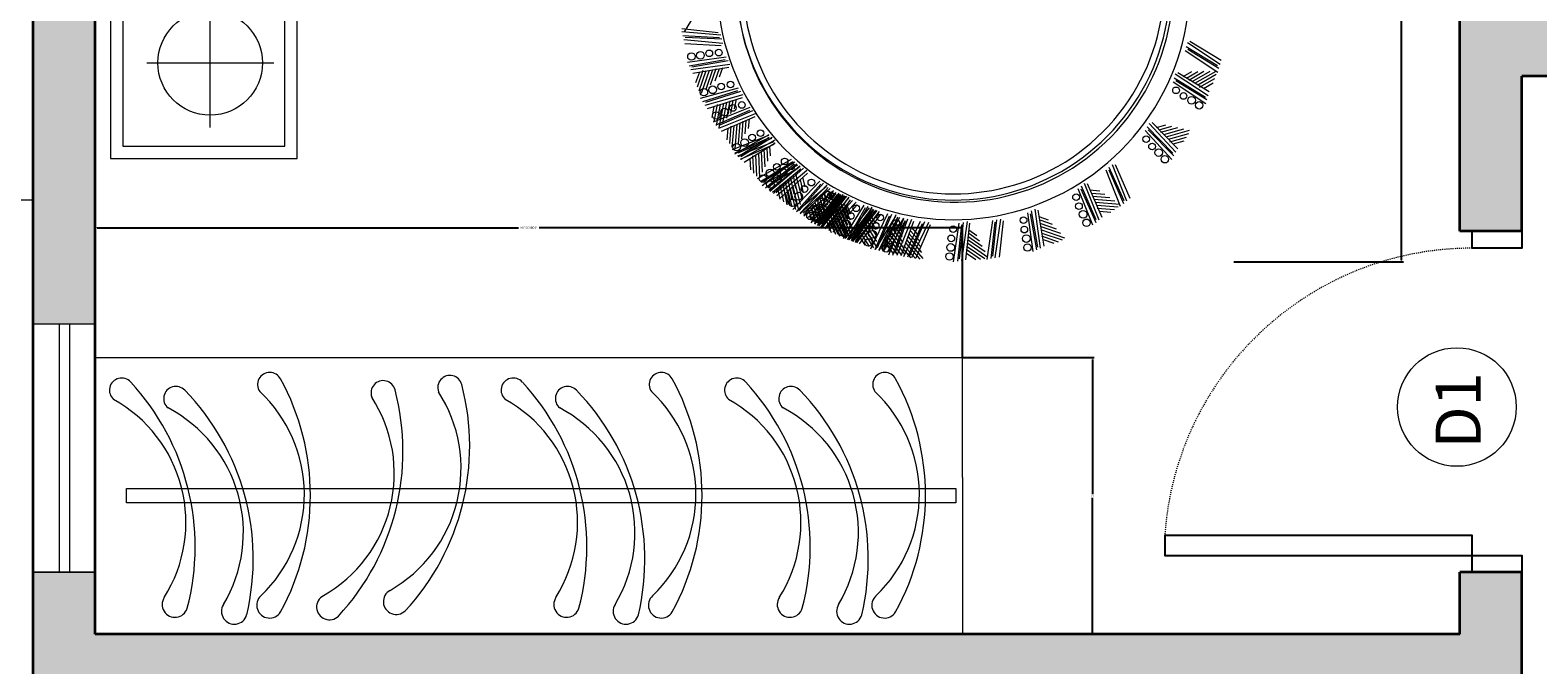
# Model space of a CAD drawing. Units: inches. Extents: x 2701 to 6846, y 811 to 2447.
# Tile 9 of 20: x 2780 to 2926, y 1309 to 1371. Entities that reach past the tile are written whole.
import ezdxf

# ---------------------------------------------------------------- set-up
doc = ezdxf.new("R2010")
doc.units = ezdxf.units.IN
doc.linetypes.add('HIDDEN4', pattern=[0.09375, 0.0625, -0.03125])
for name, color, linetype, lineweight in [('A-ANNO-DIMS', 2, 'Continuous', 18), ('A-ANNO-IDEN', 7, 'Continuous', 13), ('A-DOOR', 4, 'Continuous', 25), ('A-DOOR-SWNG', 4, 'HIDDEN4', 13), ('A-FLOR-PATT', 252, 'Continuous', 13), ('A-FURN', 8, 'Continuous', 13), ('A-GLAZ', 4, 'Continuous', 18), ('A-WALL', 7, 'Continuous', 35)]:
    doc.layers.add(name, color=color, linetype=linetype, lineweight=lineweight)
doc.layers.add('A-WALL-PATT', color=18, linetype='Continuous', lineweight=13, true_color=0x000000)
doc.styles.add('DIM_FONT', font='SIMPLEX.shx', dxfattribs={"width": 0.8})
doc.styles.get("Standard").update_dxf_attribs({"font": 'arial.ttf'})
doc.dimstyles.get("Standard").update_dxf_attribs({"dimtxt": 0.18, "dimasz": 0.18, "dimexe": 0.18, "dimexo": 0.0625, "dimgap": 0.09, "dimtad": 0, "dimtih": 1, "dimtoh": 1, "dimdec": 4, "dimzin": 0, "dimdsep": 46, "dimtxsty": 'Standard', "dimcen": 0.09, "dimadec": 0, "dimazin": 0, "dimtfac": 1, "dimtdec": 4, "dimtofl": 0, "dimtmove": 0, "dimatfit": 3, "dimfxl": 1, "dimtolj": 1, "dimtzin": 0, "dimarcsym": 0})

# ---------------------------------------------------------------- blocks, each defined once
blk = doc.blocks.new('A$C187B6359')
for p, q in [((0.2493, 2.7052), (0.2493, 2.2552)), ((0.6993, 2.7052), (0.2493, 2.7052)), ((0.2793, 2.6752), (0.2793, 2.2852)), ((0.6693, 2.6752), (0.2793, 2.6752)), ((0.4797, 2.6178), (0.4797, 2.3115)), ((0.3236, 2.4648), (0.6327, 2.4648)), ((0.2493, 2.2552), (0.6993, 2.2552)), ((0.2793, 2.2852), (0.6693, 2.2852)), ((0.4729, 1.3107), (0.4877, 1.2238)), ((0.4818, 1.3151), (0.4943, 1.2215)), ((0.5264, 1.3215), (0.5217, 1.2334)), ((0.5361, 1.3238), (0.5277, 1.2297)), ((0.5421, 1.3201), (0.5374, 1.232)), ((0.5458, 1.3261), (0.5411, 1.238)), ((0.5555, 1.3284), (0.5471, 1.2343)), ((0.5629, 1.3285), (0.5533, 1.2408)), ((0.6047, 1.292), (0.5545, 1.3229)), ((0.3781, 1.2719), (0.4034, 1.1809)), ((0.3863, 1.2774), (0.413, 1.1934)), ((0.3946, 1.283), (0.4199, 1.192)), ((0.4617, 1.2625), (0.406, 1.2816)), ((0.4604, 1.2704), (0.4117, 1.2871)), ((0.4614, 1.2774), (0.4216, 1.2911)), ((0.4577, 1.2862), (0.4318, 1.2951)), ((0.455, 1.302), (0.4698, 1.215)), ((0.4639, 1.3064), (0.4764, 1.2128)), ((0.4706, 1.3041), (0.4854, 1.2171)), ((0.3226, 1.2389), (0.3575, 1.1512)), ((0.3819, 1.2281), (0.3242, 1.2393)), ((0.3795, 1.2357), (0.3291, 1.2455)), ((0.3296, 1.2383), (0.3651, 1.1576)), ((0.3302, 1.2453), (0.3657, 1.1646)), ((0.3378, 1.2518), (0.3728, 1.164)), ((0.3796, 1.2429), (0.3383, 1.2509)), ((0.3747, 1.251), (0.3478, 1.2562)), ((0.3698, 1.2663), (0.3965, 1.1822)), ((0.385, 1.2705), (0.4116, 1.1864)), ((0.4631, 1.2546), (0.4159, 1.2708)), ((0.4656, 1.2462), (0.4257, 1.2599)), ((0.4657, 1.2388), (0.4355, 1.2491)), ((0.4677, 1.2306), (0.4454, 1.2383)), ((0.2607, 1.2004), (0.3074, 1.1183)), ((0.2632, 1.1997), (0.2988, 1.1189)), ((0.2708, 1.2061), (0.3058, 1.1184)), ((0.3311, 1.1958), (0.2725, 1.2008)), ((0.3279, 1.2031), (0.2767, 1.2075)), ((0.3272, 1.2103), (0.2853, 1.2138)), ((0.3214, 1.2178), (0.2942, 1.2201)), ((0.315, 1.2325), (0.3505, 1.1518)), ((0.3844, 1.2204), (0.3354, 1.23)), ((0.388, 1.2125), (0.3466, 1.2206)), ((0.3892, 1.2052), (0.3578, 1.2113)), ((0.3923, 1.1974), (0.3691, 1.2019)), ((0.2492, 1.1645), (0.2218, 1.163)), ((0.2407, 1.1781), (0.2871, 1.1031)), ((0.2474, 1.1856), (0.2941, 1.1035)), ((0.248, 1.1868), (0.2836, 1.1061)), ((0.254, 1.193), (0.3004, 1.1179)), ((0.2544, 1.1859), (0.3008, 1.1109)), ((0.2556, 1.1933), (0.2906, 1.1055)), ((0.2626, 1.1927), (0.2982, 1.1119)), ((0.3344, 1.1885), (0.2846, 1.1927)), ((0.3389, 1.181), (0.2968, 1.1846)), ((0.3408, 1.1738), (0.309, 1.1765)), ((0.3447, 1.1664), (0.3212, 1.1684)), ((0.1789, 1.1264), (0.2352, 1.0585)), ((0.1845, 1.1347), (0.2421, 1.0599)), ((0.1874, 1.1311), (0.2341, 1.049)), ((0.194, 1.1385), (0.2404, 1.0634)), ((0.1944, 1.1315), (0.2408, 1.0564)), ((0.2007, 1.1459), (0.2474, 1.0638)), ((0.2618, 1.144), (0.203, 1.1409)), ((0.2576, 1.1509), (0.2063, 1.1481)), ((0.2559, 1.1578), (0.2139, 1.1555)), ((0.266, 1.1372), (0.2162, 1.1345)), ((0.2715, 1.1305), (0.2294, 1.1282)), ((0.1856, 1.0919), (0.1444, 1.0838)), ((0.178, 1.0976), (0.1512, 1.0923)), ((0.1547, 1.0907), (0.2141, 1.0255)), ((0.1599, 1.0992), (0.2209, 1.0271)), ((0.1651, 1.1077), (0.2244, 1.0425)), ((0.1667, 1.1009), (0.2261, 1.0356)), ((0.1678, 1.1099), (0.2241, 1.042)), ((0.1703, 1.1162), (0.2313, 1.0441)), ((0.1733, 1.1182), (0.231, 1.0434)), ((0.1802, 1.1195), (0.2366, 1.0516)), ((0.1807, 1.1237), (0.2271, 1.0486)), ((0.2744, 1.1236), (0.2425, 1.1218)), ((0.2793, 1.1168), (0.2557, 1.1155)), ((0.1817, 1.0611), (0.1245, 1.0471)), ((0.1261, 1.0612), (0.1943, 0.9959)), ((0.1763, 1.067), (0.1264, 1.0548)), ((0.1734, 1.0735), (0.1325, 1.0636)), ((0.1934, 1.0791), (0.1356, 1.0678)), ((0.1882, 1.0852), (0.1378, 1.0754)), ((0.1871, 1.0551), (0.1386, 1.0433)), ((0.1655, 1.0789), (0.1389, 1.0724)), ((0.1985, 1.0729), (0.1495, 1.0633)), ((0.2049, 1.067), (0.1634, 1.0589)), ((0.2087, 1.0605), (0.1774, 1.0544)), ((0.2145, 1.0545), (0.1913, 1.05)), ((0.1337, 1.0191), (0.0941, 1.0049)), ((0.1253, 1.0235), (0.0995, 1.0143)), ((0.1057, 1.0262), (0.1651, 0.9609)), ((0.1109, 1.0347), (0.1719, 0.9626)), ((0.1133, 1.0342), (0.1792, 0.9755)), ((0.1161, 1.0432), (0.1754, 0.9779)), ((0.1176, 1.0432), (0.1858, 0.9779)), ((0.1178, 1.0363), (0.1771, 0.9711)), ((0.1213, 1.0517), (0.1823, 0.9796)), ((0.1218, 1.0522), (0.1877, 0.9935)), ((0.1242, 1.0456), (0.1901, 0.9869)), ((0.1937, 1.0495), (0.1527, 1.0395)), ((0.1979, 1.0433), (0.1668, 1.0357)), ((0.2039, 1.0375), (0.181, 1.0319)), ((0.0799, 0.9828), (0.1458, 0.9242)), ((0.0814, 0.983), (0.1561, 0.9253)), ((0.0835, 0.9891), (0.1533, 0.9352)), ((0.0842, 0.9918), (0.1524, 0.9266)), ((0.0847, 0.9924), (0.1563, 0.941)), ((0.0847, 0.9891), (0.1588, 0.9306)), ((0.0871, 0.9983), (0.1598, 0.938)), ((0.0877, 0.9861), (0.1594, 0.9347)), ((0.1433, 1.0075), (0.0879, 0.9877)), ((0.0879, 1.0018), (0.1627, 0.9441)), ((0.088, 0.9985), (0.1592, 0.9463)), ((0.1373, 1.0129), (0.0889, 0.9955)), ((0.0907, 1.0076), (0.1605, 0.9537)), ((0.091, 0.9921), (0.1622, 0.94)), ((0.0914, 1.0078), (0.1656, 0.9493)), ((0.0935, 1.0012), (0.1634, 0.9473)), ((0.0943, 1.0169), (0.167, 0.9566)), ((0.1493, 1.0022), (0.1023, 0.9854)), ((0.1564, 0.9973), (0.1167, 0.9831)), ((0.1612, 0.9915), (0.1312, 0.9808)), ((0.1678, 0.9864), (0.1456, 0.9784)), ((0.1107, 0.9503), (0.0577, 0.9247)), ((0.1042, 0.9549), (0.0579, 0.9326)), ((0.1136, 0.956), (0.0603, 0.931)), ((0.1071, 0.9608), (0.0606, 0.9389)), ((0.1152, 0.9646), (0.0614, 0.9409)), ((0.1089, 0.9695), (0.0618, 0.9488)), ((0.0999, 0.9607), (0.0621, 0.9424)), ((0.103, 0.9666), (0.0649, 0.9487)), ((0.1049, 0.9754), (0.0664, 0.9585)), ((0.0911, 0.9643), (0.0665, 0.9524)), ((0.0942, 0.9703), (0.0694, 0.9586)), ((0.0962, 0.9793), (0.0711, 0.9683)), ((0.0714, 0.9648), (0.1373, 0.9062)), ((0.1172, 0.9456), (0.0723, 0.9239)), ((0.1201, 0.9513), (0.0749, 0.9301)), ((0.0756, 0.9738), (0.1439, 0.9085)), ((0.1216, 0.9597), (0.0759, 0.9396)), ((0.0781, 0.9736), (0.1498, 0.9222)), ((0.0813, 0.9797), (0.1524, 0.9276)), ((0.0823, 0.9762), (0.1482, 0.9175)), ((0.1277, 0.9471), (0.0895, 0.9292)), ((0.1291, 0.9553), (0.0905, 0.9383)), ((0.1343, 0.9499), (0.105, 0.937)), ((0.1412, 0.9452), (0.1196, 0.9357)), ((0.047, 0.9096), (0.1217, 0.8519)), ((0.0494, 0.9097), (0.1261, 0.8661)), ((0.0495, 0.9161), (0.1236, 0.8576)), ((0.0503, 0.919), (0.122, 0.8676)), ((0.0517, 0.9194), (0.1321, 0.8698)), ((0.0529, 0.9254), (0.124, 0.8733)), ((0.0533, 0.9127), (0.125, 0.8613)), ((0.0535, 0.9284), (0.1283, 0.8707)), ((0.054, 0.9291), (0.1307, 0.8855)), ((0.0559, 0.9191), (0.127, 0.8669)), ((0.0563, 0.9387), (0.1367, 0.8892)), ((0.0563, 0.9348), (0.1304, 0.8763)), ((0.0577, 0.9231), (0.1344, 0.8795)), ((0.1249, 0.9415), (0.0869, 0.9231)), ((0.1302, 0.9362), (0.1015, 0.9224)), ((0.133, 0.9418), (0.1041, 0.9282)), ((0.1373, 0.9318), (0.116, 0.9216)), ((0.1401, 0.9374), (0.1187, 0.9273)), ((0.0314, 0.8727), (0.1166, 0.8319)), ((0.0773, 0.8938), (0.0336, 0.8667)), ((0.0843, 0.8899), (0.0343, 0.8589)), ((0.0725, 0.8991), (0.0368, 0.877)), ((0.0634, 0.9017), (0.0401, 0.8873)), ((0.0437, 0.9002), (0.1154, 0.8488)), ((0.0461, 0.9067), (0.1173, 0.8546)), ((0.0913, 0.8859), (0.0489, 0.8596)), ((0.0993, 0.8826), (0.0635, 0.8604)), ((0.1052, 0.878), (0.0781, 0.8612)), ((0.1127, 0.8744), (0.0927, 0.8619)), ((0.0424, 0.8367), (0.0208, 0.8199)), ((0.0252, 0.8428), (0.1056, 0.7932)), ((0.0275, 0.8525), (0.1042, 0.8089)), ((0.0277, 0.8431), (0.1085, 0.8078)), ((0.0289, 0.8529), (0.1141, 0.8121)), ((0.0298, 0.8621), (0.1102, 0.8126)), ((0.0301, 0.8628), (0.111, 0.8276)), ((0.0312, 0.8465), (0.1079, 0.8029)), ((0.0345, 0.8573), (0.1153, 0.822)), ((0.0151, 0.8), (0.0978, 0.7693)), ((0.0158, 0.8099), (0.1031, 0.774)), ((0.0571, 0.8302), (0.0165, 0.7987)), ((0.0165, 0.8199), (0.0992, 0.7892)), ((0.0171, 0.8298), (0.1045, 0.7938)), ((0.0644, 0.827), (0.0179, 0.7909)), ((0.0517, 0.835), (0.0185, 0.8092)), ((0.0211, 0.8145), (0.1038, 0.7839)), ((0.023, 0.8331), (0.0997, 0.7895)), ((0.0718, 0.8238), (0.0324, 0.7932)), ((0.0801, 0.8214), (0.0468, 0.7955)), ((0.0865, 0.8174), (0.0612, 0.7978)), ((0.0943, 0.8146), (0.0757, 0.8001)), ((0.0452, 0.7888), (0.0064, 0.7551)), ((0.0396, 0.7933), (0.0079, 0.7657)), ((0.0527, 0.7861), (0.0083, 0.7474)), ((0.0094, 0.7641), (0.0902, 0.7289)), ((0.0301, 0.7944), (0.0095, 0.7765)), ((0.0106, 0.774), (0.0958, 0.7332)), ((0.0119, 0.7839), (0.0927, 0.7486)), ((0.0131, 0.7937), (0.0983, 0.7529)), ((0.0162, 0.7783), (0.0971, 0.743)), ((0.0602, 0.7833), (0.0226, 0.7505)), ((0.0687, 0.7813), (0.0369, 0.7536)), ((0.0752, 0.7777), (0.0512, 0.7567)), ((0.0832, 0.7753), (0.0654, 0.7598)), ((0, 0.6734), (0.0935, 0.6598)), ((0.0018, 0.6636), (0.0894, 0.654)), ((0.0075, 0.6596), (0.0952, 0.65)), ((0.0035, 0.6538), (0.097, 0.6402)), ((0.0053, 0.644), (0.093, 0.6344)), ((0.0212, 0.6423), (0.0056, 0.6198)), ((0.0306, 0.6435), (0.0066, 0.609)), ((0.0372, 0.6405), (0.0078, 0.5983)), ((0.0451, 0.6396), (0.0115, 0.5913)), ((0.0531, 0.6388), (0.0246, 0.5978)), ((0.0618, 0.639), (0.0377, 0.6043)), ((0.069, 0.637), (0.0508, 0.6108)), ((0.0774, 0.6367), (0.0639, 0.6173)), ((0.0061, 0.5926), (0.0995, 0.579)), ((0.0078, 0.5828), (0.0955, 0.5732)), ((0.0096, 0.573), (0.1031, 0.5594)), ((0.0113, 0.5632), (0.099, 0.5536)), ((0.0136, 0.5788), (0.1013, 0.5692)), ((0.0247, 0.4821), (0.1183, 0.4946)), ((0.0291, 0.4731), (0.116, 0.4879)), ((0.0334, 0.4642), (0.1271, 0.4767)), ((0.0357, 0.4708), (0.1227, 0.4857)), ((0.0378, 0.4552), (0.1248, 0.47)), ((0.0536, 0.4579), (0.0448, 0.4321)), ((0.0624, 0.4617), (0.0487, 0.4219)), ((0.0694, 0.4606), (0.0528, 0.412)), ((0.0773, 0.462), (0.0582, 0.4063)), ((0.0853, 0.4633), (0.0691, 0.4161)), ((0.0936, 0.4659), (0.0799, 0.426)), ((0.1011, 0.466), (0.0907, 0.4358)), ((0.1092, 0.468), (0.1015, 0.4456)), ((0.0881, 0.3381), (0.1758, 0.373)), ((0.0945, 0.3304), (0.1752, 0.366)), ((0.1015, 0.3299), (0.1822, 0.3654)), ((0.1009, 0.3228), (0.1886, 0.3578)), ((0.1073, 0.3152), (0.188, 0.3508)), ((0.1296, 0.3275), (0.126, 0.2856)), ((0.1367, 0.3282), (0.1323, 0.2769)), ((0.144, 0.3314), (0.139, 0.2727)), ((0.1514, 0.3346), (0.1471, 0.2849)), ((0.1588, 0.3391), (0.1552, 0.2971)), ((0.166, 0.3411), (0.1633, 0.3093)), ((0.1734, 0.345), (0.1714, 0.3214)), ((0.122, 0.3217), (0.1197, 0.2944)), ((0.1337, 0.2711), (0.2215, 0.3061)), ((0.1401, 0.2635), (0.2209, 0.299)), ((0.1466, 0.2559), (0.2343, 0.2908)), ((0.1472, 0.2629), (0.2279, 0.2985)), ((0.153, 0.2483), (0.2337, 0.2838)), ((0.2468, 0.148), (0.3166, 0.2116)), ((0.2555, 0.1431), (0.3185, 0.2048)), ((0.2623, 0.145), (0.3253, 0.2068)), ((0.2642, 0.1382), (0.334, 0.2019)), ((0.2729, 0.1334), (0.3359, 0.1951)), ((0.3243, 0.1845), (0.3307, 0.1618)), ((0.2894, 0.1527), (0.3008, 0.1122)), ((0.2958, 0.1558), (0.3098, 0.1064)), ((0.3015, 0.1614), (0.3176, 0.1048)), ((0.3073, 0.1671), (0.3208, 0.1191)), ((0.3126, 0.1739), (0.3241, 0.1333)), ((0.3187, 0.1783), (0.3274, 0.1475)), ((0.2843, 0.1446), (0.2918, 0.1183)), ((0.3809, 0.0657), (0.4331, 0.1445)), ((0.3906, 0.0631), (0.4366, 0.1384)), ((0.3967, 0.0666), (0.4427, 0.1419)), ((0.4002, 0.0605), (0.4524, 0.1393)), ((0.4098, 0.0579), (0.4559, 0.1332)), ((0.4433, 0.1127), (0.4592, 0.085)), ((0.4472, 0.12), (0.4589, 0.0996)), ((0.4566, 0.0367), (0.5088, 0.1155)), ((0.4662, 0.0341), (0.5123, 0.1094)), ((0.4723, 0.0377), (0.5184, 0.1129)), ((0.4759, 0.0315), (0.528, 0.1103)), ((0.4211, 0.0807), (0.442, 0.0442)), ((0.4265, 0.0853), (0.4522, 0.0407)), ((0.4307, 0.0921), (0.4601, 0.0411)), ((0.4349, 0.099), (0.4598, 0.0557)), ((0.4385, 0.1069), (0.4595, 0.0703)), ((0.4855, 0.029), (0.5315, 0.1042)), ((0.4182, 0.0716), (0.4318, 0.0479))]:
    blk.add_line(p, q)
for centre, radius in [((0.4797, 2.4648), 0.126), ((0.495, 1.3053), 0.00895), ((0.409, 1.2751), 0.00895), ((0.4979, 1.2836), 0.00929), ((0.353, 1.2454), 0.00895), ((0.4149, 1.254), 0.00929), ((0.4227, 1.2335), 0.00801), ((0.5028, 1.2622), 0.00801), ((0.5045, 1.2395), 0.00801), ((0.2766, 1.1962), 0.00895), ((0.3611, 1.2251), 0.00929), ((0.3711, 1.2055), 0.00801), ((0.4275, 1.2112), 0.00801), ((0.2875, 1.1772), 0.00929), ((0.3, 1.1592), 0.00801), ((0.3783, 1.184), 0.00801), ((0.2008, 1.1328), 0.00895), ((0.3101, 1.1388), 0.00801), ((0.1867, 1.1151), 0.00895), ((0.2008, 1.0984), 0.00929), ((0.2142, 1.1155), 0.00929), ((0.2165, 1.083), 0.00801), ((0.2291, 1.0994), 0.00801), ((0.1426, 1.0618), 0.00895), ((0.1584, 1.0467), 0.00929), ((0.2301, 1.0648), 0.00801), ((0.2419, 1.0806), 0.00801), ((0.1078, 1.01), 0.00895), ((0.1107, 1.0186), 0.00895), ((0.1756, 1.033), 0.00801), ((0.1911, 1.0163), 0.00801), ((0.1043, 1.0041), 0.00895), ((0.1216, 0.9908), 0.00929), ((0.1249, 0.9964), 0.00929), ((0.1276, 1.0047), 0.00929), ((0.1401, 0.979), 0.00801), ((0.1434, 0.9844), 0.00801), ((0.1457, 0.9922), 0.00801), ((0.1623, 0.9767), 0.00801), ((0.0722, 0.9428), 0.00895), ((0.1573, 0.964), 0.00801), ((0.1604, 0.9693), 0.00801), ((0.0909, 0.9313), 0.00929), ((0.1106, 0.9215), 0.00801), ((0.1292, 0.9085), 0.00801), ((0.0469, 0.8784), 0.00895), ((0.0666, 0.8689), 0.00929), ((0.0323, 0.8363), 0.00895), ((0.0525, 0.828), 0.00929), ((0.0872, 0.8613), 0.00801), ((0.1071, 0.8503), 0.00801), ((0.0735, 0.8215), 0.00801), ((0.094, 0.8117), 0.00801), ((0.0131, 0.6834), 0.00895), ((0.0347, 0.6803), 0.00929), ((0.0567, 0.6791), 0.00801), ((0.079, 0.6745), 0.00801), ((0.0777, 0.5031), 0.00801), ((0.1003, 0.5048), 0.00801), ((0.0345, 0.4953), 0.00895), ((0.0562, 0.4982), 0.00929), ((0.1147, 0.3614), 0.00929), ((0.1343, 0.3714), 0.00801), ((0.1559, 0.3785), 0.00801), ((0.0944, 0.3533), 0.00895), ((0.2635, 0.1792), 0.00929), ((0.2784, 0.1954), 0.00801), ((0.296, 0.2097), 0.00801), ((0.2474, 0.1644), 0.00895), ((0.4136, 0.1376), 0.00801), ((0.3895, 0.1001), 0.00929), ((0.4, 0.1194), 0.00801), ((0.3775, 0.0818), 0.00895)]:
    blk.add_circle(centre, radius)
for centre, radius, start, end in [((0.6715, 0.6736), 0.5699, 87.1307, 3.1127), ((0.6698, 0.67), 0.5261, 86.7143, 0.065), ((0.6715, 0.6736), 0.5225, 86.8806, 3.3918), ((0.6715, 0.6735), 0.5076, 86.694, 3.4914)]:
    blk.add_arc(centre, radius, start, end)
at = {"style": 'DIM_FONT', "text_generation_flag": 4, "width": 0.8, "flags": 9}
for tag in ['YSIZE', 'XSIZE']:
    blk.add_attdef(tag, (2.1999, 2.7053), '', height=0.0005, rotation=180, dxfattribs=at)
blk = doc.blocks.new('A$C20D7642B')
for p, q in [((0, 1879.7), (0, 0)), ((600, 1879.7), (0, 1879.7)), ((600, 1879.7), (600, 0)), ((285.2, 14), (285.2, 1812.3)), ((285.2, 1812.3), (316, 1812.3)), ((316, 1812.3), (316, 14)), ((340, 0), (0, 0)), ((316, 14), (285.2, 14)), ((340, 0), (600, 0))]:
    blk.add_line(p, q)
for centre, radius, start, end in [((242.6, 1988.3), 305.1, 237.7855, 330.9171), ((529.2, 1822.6), 26.4, 312.0689, 138.8769), ((189.7, 2189.4), 526.2, 255.3064, 312.7492), ((64.5, 1707), 27.8, 56.3378, 252.7376), ((220.7, 1863.8), 305.1, 239.1708, 332.3023), ((511.2, 1705.1), 26.4, 313.4541, 140.2621), ((163, 2063.5), 526.2, 256.6916, 314.1345), ((49.5, 1578.3), 27.8, 57.7231, 254.1228), ((62.8, 1501.9), 27.8, 42.31, 238.7098), ((303.8, 1731.6), 305.1, 223.7577, 316.8893), ((541.6, 1501.4), 26.4, 298.0411, 124.849), ((301.2, 1939.5), 526.2, 241.2786, 298.7214), ((59.1, 1372.1), 27.8, 28.2801, 224.6799), ((348.6, 1536.6), 305.1, 209.7278, 302.8594), ((396.5, 1738.9), 526.2, 227.2487, 284.6915), ((523.6, 1255.6), 26.4, 284.0112, 110.8192), ((70.6, 1227.4), 27.8, 28.2801, 224.6799), ((360, 1391.9), 305.1, 209.7278, 302.8594), ((408, 1594.2), 526.2, 227.2487, 284.6915), ((535, 1110.9), 26.4, 284.0112, 110.8192), ((242.6, 1139.3), 305.1, 237.7855, 330.9171), ((529.2, 973.6), 26.4, 312.0689, 138.8769), ((189.7, 1340.3), 526.2, 255.3064, 312.7492), ((64.5, 857.9), 27.8, 56.3378, 252.7376), ((511.2, 856), 26.4, 313.4541, 140.2621), ((220.7, 1014.8), 305.1, 239.1708, 332.3023), ((163, 1214.5), 526.2, 256.6916, 314.1345), ((49.5, 729.2), 27.8, 57.7231, 254.1228), ((62.8, 652.8), 27.8, 42.31, 238.7098), ((303.8, 882.6), 305.1, 223.7577, 316.8893), ((541.6, 652.4), 26.4, 298.0411, 124.849), ((301.2, 1090.5), 526.2, 241.2786, 298.7214), ((242.6, 655), 305.1, 237.7855, 330.9171), ((529.2, 489.2), 26.4, 312.0689, 138.8769), ((189.7, 856), 526.2, 255.3064, 312.7492), ((64.5, 373.6), 27.8, 56.3378, 252.7376), ((511.2, 371.7), 26.4, 313.4541, 140.2621), ((220.7, 530.5), 305.1, 239.1708, 332.3023), ((163, 730.2), 526.2, 256.6916, 314.1345), ((49.5, 244.9), 27.8, 57.7231, 254.1228), ((62.8, 168.5), 27.8, 42.31, 238.7098), ((303.8, 398.3), 305.1, 223.7577, 316.8893), ((541.6, 168), 26.4, 298.0411, 124.849), ((301.2, 606.1), 526.2, 241.2786, 298.7214)]:
    blk.add_arc(centre, radius, start, end)
blk = doc.blocks.new('DOOR-D1-33IN-PANEL-FRAME')
blk.add_lwpolyline([(0, 33), (0, 31.37), (4.8, 31.37), (4.8, 33), (0, 33)], close=True)
for points in [[(4.32, 33), (0.48, 33)], [(4.8, 0), (4.8, 3.55), (34.54, 3.55), (34.54, 1.63), (0, 1.63), (0, 0)], [(0, 0), (4.8, 0)], [(4.32, 0), (0.48, 0)]]:
    blk.add_lwpolyline(points)
blk = doc.blocks.new('WIN-W2-24IN')
for p, q in [((24, 6), (0, 6)), ((24, 6), (0, 6)), ((0, 0), (0, 6)), ((24, 6), (24, 6)), ((24, 6), (24, 0)), ((24, 3.5), (0, 3.5)), ((24, 2.5), (0, 2.5)), ((24, 0), (0, 0))]:
    blk.add_line(p, q)
blk = doc.blocks.new('*D45')
at = {"layer": 'A-ANNO-DIMS', "color": 0, "lineweight": -2, "transparency": 16777216}
for p, q in [((2785.97, 1338.89), (2785.97, 1351.58)), ((2786.15, 1351.4), (2826.91, 1351.4)), ((2869.67, 1351.4), (2828.91, 1351.4)), ((2869.85, 1338.89), (2869.85, 1351.58))]:
    blk.add_line(p, q, dxfattribs=at)
at = {"layer": 'A-ANNO-DIMS', "color": 0, "transparency": 16777216}
for points in [[(2786.15, 1351.43), (2786.15, 1351.37), (2785.97, 1351.4)], [(2869.67, 1351.43), (2869.67, 1351.37), (2869.85, 1351.4)]]:
    blk.add_solid(points, dxfattribs=at)
at = {"layer": 'Defpoints', "color": 0, "transparency": 16777216}
for p in [(2785.97, 1351.4), (2785.97, 1338.82), (2869.85, 1338.82)]:
    blk.add_point(p, dxfattribs=at)
at = {"layer": 'A-ANNO-DIMS', "color": 0, "transparency": 16777216, "insert": (2827.91, 1351.4), "char_height": 0.18, "attachment_point": 5}
blk.add_mtext('\\A1;WARDROBE 84', dxfattribs=at)
blk = doc.blocks.new('*D46')
at = {"layer": 'A-ANNO-DIMS', "color": 0, "lineweight": -2, "transparency": 16777216}
for p, q in [((2869.91, 1338.82), (2882.61, 1338.82)), ((2882.43, 1338.64), (2882.43, 1325.62)), ((2882.43, 1312.23), (2882.43, 1325.26)), ((2869.91, 1312.05), (2882.61, 1312.05))]:
    blk.add_line(p, q, dxfattribs=at)
at = {"layer": 'A-ANNO-DIMS', "color": 0, "transparency": 16777216}
for points in [[(2882.4, 1338.64), (2882.46, 1338.64), (2882.43, 1338.82)], [(2882.4, 1312.23), (2882.46, 1312.23), (2882.43, 1312.05)]]:
    blk.add_solid(points, dxfattribs=at)
at = {"layer": 'Defpoints', "color": 0, "transparency": 16777216}
for p in [(2869.85, 1338.82), (2882.43, 1338.82), (2869.85, 1312.05)]:
    blk.add_point(p, dxfattribs=at)
at = {"layer": 'A-ANNO-DIMS', "color": 0, "transparency": 16777216, "insert": (2882.43, 1325.44), "char_height": 0.18, "attachment_point": 5}
blk.add_mtext('\\A1;27', dxfattribs=at)
blk = doc.blocks.new('*D50')
at = {"layer": 'A-ANNO-DIMS', "color": 0, "lineweight": -2, "transparency": 16777216}
for p, q in [((2896.11, 1454.53), (2912.52, 1454.53)), ((2912.34, 1454.35), (2912.34, 1401.49)), ((2912.34, 1348.27), (2912.34, 1401.13)), ((2896.11, 1348.09), (2912.52, 1348.09))]:
    blk.add_line(p, q, dxfattribs=at)
at = {"layer": 'A-ANNO-DIMS', "color": 0, "transparency": 16777216}
for points in [[(2912.31, 1454.35), (2912.37, 1454.35), (2912.34, 1454.53)], [(2912.31, 1348.27), (2912.37, 1348.27), (2912.34, 1348.09)]]:
    blk.add_solid(points, dxfattribs=at)
at = {"layer": 'Defpoints', "color": 0, "transparency": 16777216}
for p in [(2896.04, 1454.53), (2912.34, 1454.53), (2896.04, 1348.09)]:
    blk.add_point(p, dxfattribs=at)
at = {"layer": 'A-ANNO-DIMS', "color": 0, "transparency": 16777216, "insert": (2912.34, 1401.31), "char_height": 0.18, "attachment_point": 5}
blk.add_mtext('\\A1;106', dxfattribs=at)

msp = doc.modelspace()

# ---------------------------------------------------------------- hatches: boundary and pattern name
at = {"layer": 'A-FLOR-PATT'}
h = msp.add_hatch(dxfattribs=at)
h.set_pattern_fill('ANGLE', color=256)
h.set_pattern_definition([(0, (0, 0), (0, 6.985), [5.08, -1.905]), (90, (0, 0), (-6.985, 4e-16), [5.08, -1.905])])
h.paths.add_polyline_path([(2841.81, 1296.51, -0.109453), (2842.61, 1300.13, -0.102375), (2844.98, 1303.3, -0.093743), (2848.43, 1305.37, -0.062463), (2851.37, 1306.05), (2785.97, 1306.05), (2785.97, 1258.05), (2827.97, 1258.05), (2827.97, 1256.41), (2829.45, 1256.41, -0.394827), (2854.75, 1283.45), (2856.49, 1283.45), (2856.49, 1256.41), (2857.97, 1256.41), (2857.97, 1258.05), (2863.97, 1258.05), (2863.97, 1306.05), (2853.87, 1306.05, -0.062463), (2856.81, 1305.37, -0.093743), (2860.26, 1303.3, -0.102375), (2862.62, 1300.13, -0.109453), (2863.42, 1296.51, -0.109453), (2862.62, 1292.89, -0.102375), (2860.26, 1289.72, -0.093738), (2856.81, 1287.65, -0.088425), (2852.62, 1286.91, -0.088425), (2848.43, 1287.65, -0.093738), (2844.98, 1289.72, -0.102375), (2842.61, 1292.89, -0.109453)])
h.paths.add_polyline_path([(2805.21, 1273.88, -0.141745), (2808.32, 1271.77, -0.184983), (2809.77, 1267.97, -0.184983), (2808.32, 1264.18, -0.141745), (2805.21, 1262.07, -0.152244), (2799.99, 1261.8, -0.025614), (2799.37, 1261.95), (2794.37, 1263.42), (2794.36, 1263.41, -0.111242), (2793.99, 1261.92, -0.033889), (2793.11, 1260.11, -0.286745), (2792.38, 1259.65), (2787.58, 1259.65, -0.414214), (2787.15, 1260.08), (2787.15, 1267.97), (2787.15, 1275.87, -0.414214), (2787.58, 1276.3), (2792.38, 1276.3, -0.286745), (2793.11, 1275.83, -0.033889), (2793.99, 1274.03, -0.105104), (2794.36, 1272.63), (2794.37, 1272.53), (2799.37, 1274, -0.025614), (2799.99, 1274.15, -0.152244)], flags=16)
h.paths.add_polyline_path([(2804.68, 1272.34, -0.144945), (2807.09, 1270.71, -0.0358), (2807.45, 1270.25, -0.133285), (2807.89, 1268.61), (2807.89, 1267.97), (2807.89, 1267.34, -0.133285), (2807.45, 1265.7, -0.0358), (2807.09, 1265.24, -0.144945), (2804.68, 1263.61, -0.155404), (2800.34, 1263.39, -0.364511), (2796.49, 1267.97, -0.364511), (2800.34, 1272.56, -0.155404)], flags=0)
h.paths.add_polyline_path([(2800.02, 1268.9, 0.169298), (2799.13, 1268.12, 0.076667), (2799.1, 1267.97, 0.076667), (2799.13, 1267.83, 0.169298), (2800.02, 1267.05, 0.305219), (2800.37, 1267.16, 0.169535), (2800.65, 1267.97, 0.169535), (2800.37, 1268.79, 0.305219)], flags=0)
h.paths.add_polyline_path([(2971.97, 1456.05), (2923.97, 1456.05), (2923.97, 1408.05), (2922.33, 1408.05), (2922.33, 1406.57, -0.394827), (2949.37, 1381.27), (2949.37, 1379.53), (2922.33, 1379.53), (2922.33, 1378.05), (2923.97, 1378.05), (2923.97, 1372.05), (2971.97, 1372.05)])
h.paths.add_polyline_path([(2939.82, 1436.53, -0.141745), (2937.71, 1433.42, -0.184983), (2933.91, 1431.97, -0.184983), (2930.12, 1433.42, -0.141745), (2928.01, 1436.53, -0.152244), (2927.74, 1441.75, -0.025614), (2927.89, 1442.37), (2929.36, 1447.38), (2929.35, 1447.38, -0.111242), (2927.86, 1447.75, -0.033889), (2926.05, 1448.63, -0.286745), (2925.59, 1449.37), (2925.59, 1454.16, -0.414214), (2926.02, 1454.59), (2933.91, 1454.59), (2941.81, 1454.59, -0.414207), (2942.24, 1454.16), (2942.24, 1449.37, -0.286745), (2941.78, 1448.63, -0.033889), (2939.97, 1447.75, -0.105104), (2938.57, 1447.38), (2938.47, 1447.38), (2939.94, 1442.37, -0.025614), (2940.09, 1441.75, -0.152244)], flags=16)
h.paths.add_polyline_path([(2938.28, 1437.06, -0.144945), (2936.65, 1434.65, -0.0358), (2936.19, 1434.29, -0.133285), (2934.55, 1433.85), (2933.91, 1433.85), (2933.28, 1433.85, -0.133285), (2931.64, 1434.29, -0.0358), (2931.18, 1434.65, -0.144945), (2929.55, 1437.06, -0.155404), (2929.33, 1441.4, -0.364511), (2933.91, 1445.26, -0.364511), (2938.5, 1441.4, -0.155404)], flags=0)
h.paths.add_polyline_path([(2969.16, 1392.04, -0.093743), (2971.22, 1388.6, -0.088421), (2971.97, 1384.4, -0.088421), (2971.22, 1380.21, -0.093743), (2969.16, 1376.76, -0.102375), (2965.99, 1374.4, -0.109453), (2962.37, 1373.6, -0.109453), (2958.75, 1374.4, -0.102375), (2955.58, 1376.76, -0.093738), (2953.51, 1380.21, -0.088425), (2952.76, 1384.4, -0.088425), (2953.51, 1388.6, -0.093738), (2955.58, 1392.04, -0.102375), (2958.75, 1394.41, -0.109453), (2962.37, 1395.21, -0.109453), (2965.99, 1394.41, -0.102375)], flags=0)
edge = h.paths.add_edge_path(flags=16)
edge.add_arc((2961.07, 1384.86), 10.2, 20.2132, 41.6336, ccw=False)
edge.add_spline(control_points=[(2970.65, 1388.38), (2970.46, 1387.83), (2970, 1386.48), (2971.44, 1384.4), (2969.87, 1382.34), (2970.41, 1381.01), (2970.65, 1380.43)], knot_values=[0, 0, 0, 0, 0.041109, 0.100337, 0.155913, 0.199586, 0.199586, 0.199586, 0.199586], degree=3, periodic=0)
edge.add_arc((2961.07, 1383.95), 10.2, 318.3664, 339.7868, ccw=False)
edge.add_arc((2961.86, 1383.25), 9.15, 294.9853, 318.3664, ccw=False)
edge.add_arc((2962.37, 1382.17), 7.95, 270, 294.9853, ccw=False)
edge.add_arc((2962.37, 1382.17), 7.95, 245.0147, 270, ccw=False)
edge.add_arc((2962.87, 1383.25), 9.15, 221.6336, 245.0147, ccw=False)
edge.add_arc((2963.66, 1383.95), 10.2, 200.213, 221.6336, ccw=False)
edge.add_arc((2964.89, 1384.4), 11.51, 180, 200.213, ccw=False)
edge.add_arc((2964.89, 1384.4), 11.51, 159.787, 180, ccw=False)
edge.add_arc((2963.66, 1384.86), 10.2, 138.3664, 159.787, ccw=False)
edge.add_arc((2962.87, 1385.56), 9.15, 114.9853, 138.3664, ccw=False)
edge.add_arc((2962.37, 1386.64), 7.95, 90, 114.9853, ccw=False)
edge.add_arc((2962.37, 1386.64), 7.95, 65.0147, 90, ccw=False)
edge.add_arc((2961.86, 1385.56), 9.15, 41.6336, 65.0147, ccw=False)
h.paths.add_polyline_path([(2963.81, 1393.33, -0.126458), (2966.61, 1390.68, -0.141697), (2967.17, 1388.76), (2967.17, 1387.41, -1), (2969.57, 1387.41, -0.414214), (2968.37, 1386.21), (2963.57, 1385, 0.146218), (2963.31, 1384.66), (2968.97, 1385.64), (2968.97, 1383.15), (2963.32, 1384.13, 0.140312), (2963.57, 1383.8), (2968.37, 1382.6, -0.414214), (2969.57, 1381.4, -1), (2967.17, 1381.4), (2967.17, 1380.04, -0.149025), (2966.56, 1378.03, -0.012759), (2966.26, 1377.62, -0.106303), (2963.81, 1375.48, -0.126822), (2961.17, 1374.8, -0.126822), (2958.52, 1375.48, -0.106303), (2956.07, 1377.62, -0.085722), (2954.54, 1380.62, -0.075351), (2953.96, 1384.4, -0.075351), (2954.54, 1388.19, -0.085722), (2956.07, 1391.19, -0.106303), (2958.52, 1393.33, -0.126822), (2961.17, 1394.01, -0.126822)], flags=0)
h.paths.add_polyline_path([(2934.84, 1441.73, 0.169298), (2934.06, 1442.61, 0.076667), (2933.91, 1442.64, 0.076667), (2933.77, 1442.61, 0.169298), (2932.99, 1441.73, 0.305219), (2933.1, 1441.38, 0.169535), (2933.91, 1441.09, 0.169535), (2934.73, 1441.38, 0.305219)], flags=0)
h.paths.add_polyline_path([(2969.32, 1387.41, -1), (2967.42, 1387.41, -1)], flags=0)
h.paths.add_polyline_path([(2968.83, 1387.41, -1), (2967.91, 1387.41, -1)], flags=0)
h.paths.add_polyline_path([(2962.13, 1384.36, -1), (2960.21, 1384.36, -1)], flags=0)
h.paths.add_polyline_path([(2961.8, 1384.36, -1), (2960.54, 1384.36, -1)], flags=0)
h.paths.add_polyline_path([(2969.32, 1381.4, -1), (2967.42, 1381.4, -1)], flags=0)
h.paths.add_polyline_path([(2968.83, 1381.4, -1), (2967.91, 1381.4, -1)], flags=0)
h.paths.add_polyline_path([(3085.97, 1306.05), (3001.97, 1306.05), (3001.97, 1300.05), (3000.33, 1300.05), (3000.33, 1298.57), (3027.37, 1298.57), (3027.37, 1296.83, -0.394827), (3000.33, 1271.53), (3000.33, 1270.05), (3001.97, 1270.05), (3001.97, 1258.05), (3085.97, 1258.05)])
h.paths.add_polyline_path([(3033.33, 1274.44, -0.102375), (3035.7, 1271.27, -0.109453), (3036.5, 1267.65, -0.109453), (3035.7, 1264.04, -0.102375), (3033.33, 1260.86, -0.093743), (3029.88, 1258.8, -0.088421), (3025.69, 1258.05, -0.088421), (3021.5, 1258.8, -0.093743), (3018.05, 1260.86, -0.102375), (3015.69, 1264.04, -0.109453), (3014.89, 1267.65, -0.109453), (3015.69, 1271.27, -0.102375), (3018.05, 1274.44, -0.093738), (3021.5, 1276.51, -0.088425), (3025.69, 1277.26, -0.088425), (3029.88, 1276.51, -0.093738)], flags=0)
edge = h.paths.add_edge_path(flags=16)
edge.add_arc((3026.85, 1267.15), 9.15, 24.9853, 48.3664, ccw=False)
edge.add_arc((3027.93, 1267.65), 7.95, 0, 24.9853, ccw=False)
edge.add_arc((3027.93, 1267.65), 7.95, -24.9853, 0, ccw=False)
edge.add_arc((3026.85, 1268.16), 9.15, 311.6336, 335.0147, ccw=False)
edge.add_arc((3026.15, 1268.95), 10.2, 290.2132, 311.6336, ccw=False)
edge.add_spline(control_points=[(3029.67, 1259.38), (3029.09, 1259.61), (3027.76, 1260.15), (3025.7, 1258.59), (3023.62, 1260.02), (3022.27, 1259.56), (3021.71, 1259.38)], knot_values=[0, 0, 0, 0, 0.043673, 0.099248, 0.158477, 0.199586, 0.199586, 0.199586, 0.199586], degree=3, periodic=0)
edge.add_arc((3025.24, 1268.95), 10.2, 228.3664, 249.7868, ccw=False)
edge.add_arc((3024.54, 1268.16), 9.15, 204.9853, 228.3664, ccw=False)
edge.add_arc((3023.45, 1267.65), 7.95, 180, 204.9853, ccw=False)
edge.add_arc((3023.45, 1267.65), 7.95, 155.0147, 180, ccw=False)
edge.add_arc((3024.54, 1267.15), 9.15, 131.6336, 155.0147, ccw=False)
edge.add_arc((3025.24, 1266.36), 10.2, 110.213, 131.6336, ccw=False)
edge.add_arc((3025.69, 1265.13), 11.51, 90, 110.213, ccw=False)
edge.add_arc((3025.69, 1265.13), 11.51, 69.787, 90, ccw=False)
edge.add_arc((3026.15, 1266.36), 10.2, 48.3664, 69.787, ccw=False)
h.paths.add_polyline_path([(3032.48, 1273.95, -0.106303), (3034.62, 1271.5, -0.126822), (3035.3, 1268.85, -0.126822), (3034.62, 1266.21, -0.106303), (3032.48, 1263.76, -0.012759), (3032.07, 1263.46, -0.149025), (3030.06, 1262.85), (3028.69, 1262.85, -0.414214), (3029.89, 1261.65, -1), (3027.49, 1261.65), (3026.29, 1266.45, 0.140312), (3025.97, 1266.7), (3026.94, 1261.05), (3024.46, 1261.05), (3025.43, 1266.71, 0.146218), (3025.09, 1266.45), (3023.89, 1261.65, -1), (3021.49, 1261.65, -0.414214), (3022.69, 1262.85), (3021.34, 1262.85, -0.141697), (3019.41, 1263.41, -0.126458), (3016.77, 1266.21, -0.126822), (3016.09, 1268.85, -0.126822), (3016.77, 1271.5, -0.106303), (3018.91, 1273.95, -0.085722), (3021.91, 1275.48, -0.075351), (3025.69, 1276.06, -0.075351), (3029.47, 1275.48, -0.085722)], flags=0)
h.paths.add_polyline_path([(3072.36, 1280, -0.184983), (3076.16, 1281.46, -0.184983), (3079.96, 1280, -0.141745), (3082.07, 1276.9, -0.152244), (3082.34, 1271.68, -0.025614), (3082.19, 1271.05), (3080.72, 1266.05), (3080.82, 1266.04, -0.105104), (3082.22, 1265.68, -0.033889), (3084.02, 1264.8, -0.286745), (3084.49, 1264.06), (3084.49, 1259.26, -0.41422), (3084.06, 1258.84), (3076.16, 1258.84), (3068.27, 1258.84, -0.414214), (3067.84, 1259.26), (3067.84, 1264.06, -0.286745), (3068.3, 1264.8, -0.033889), (3070.1, 1265.68, -0.105104), (3071.51, 1266.04), (3071.61, 1266.05), (3070.13, 1271.05, -0.025614), (3069.98, 1271.68, -0.152244), (3070.26, 1276.9, -0.141745)], flags=16)
h.paths.add_polyline_path([(3073.43, 1278.77, -0.0358), (3073.88, 1279.13, -0.133285), (3075.53, 1279.58), (3076.16, 1279.58), (3076.8, 1279.58, -0.133285), (3078.44, 1279.13, -0.0358), (3078.9, 1278.77, -0.144945), (3080.53, 1276.36, -0.155404), (3080.75, 1272.03, -0.364511), (3076.16, 1268.17, -0.364511), (3071.57, 1272.03, -0.155404), (3071.8, 1276.36, -0.144945)], flags=0)
h.paths.add_polyline_path([(3026.7, 1268.85, -1), (3024.78, 1268.85, -1)], flags=0)
h.paths.add_polyline_path([(3026.37, 1268.85, -1), (3025.11, 1268.85, -1)], flags=0)
h.paths.add_polyline_path([(3075.27, 1271.62, 0.157677), (3076.02, 1270.81, 0.076667), (3076.16, 1270.78, 0.076667), (3076.3, 1270.81, 0.157677), (3077.06, 1271.62, 0.374626), (3076.98, 1272.05, 0.169535), (3076.16, 1272.33, 0.169535), (3075.35, 1272.05, 0.374626)], flags=0)
h.paths.add_polyline_path([(3029.65, 1261.65, -1), (3027.74, 1261.65, -1)], flags=0)
h.paths.add_polyline_path([(3029.15, 1261.65, -1), (3028.23, 1261.65, -1)], flags=0)
h.paths.add_polyline_path([(3023.65, 1261.65, -1), (3021.74, 1261.65, -1)], flags=0)
h.paths.add_polyline_path([(3023.15, 1261.65, -1), (3022.23, 1261.65, -1)], flags=0)
h.paths.add_polyline_path([(2810.57, 1281.22), (2833.31, 1281.22), (2833.31, 1296.43), (2810.57, 1296.43)], flags=24)
h.paths.add_polyline_path([(2937.55, 1410.24), (2960.21, 1410.24), (2960.21, 1425.45), (2937.55, 1425.45)], flags=24)
h.paths.add_polyline_path([(3043.23, 1273.1), (3065.89, 1273.1), (3065.89, 1288.31), (3043.23, 1288.31)], flags=24)
at = {"layer": 'A-WALL-PATT'}
h = msp.add_hatch(color=256, dxfattribs=at)
h.dxf.hatch_style = 1
h.paths.add_polyline_path([(3085.97, 1456.05), (3085.97, 1348.05), (3091.97, 1348.05), (3091.97, 1360.05), (3091.97, 1462.05), (2960.09, 1462.05), (2960.09, 1456.05), (2971.97, 1456.05), (2971.97, 1372.05), (2923.97, 1372.05), (2923.97, 1378.05), (2917.97, 1378.05), (2917.97, 1351.05), (2923.97, 1351.05), (2923.97, 1366.05), (2971.97, 1366.05), (2971.97, 1351.05), (2976.77, 1351.05), (2977.97, 1351.05), (2977.97, 1456.05)])
h.paths.add_polyline_path([(2779.97, 1462.05), (2779.97, 1342.05), (2785.97, 1342.05), (2785.97, 1456.05), (2917.97, 1456.05), (2917.97, 1408.05), (2922.33, 1408.05), (2923.97, 1408.05), (2923.97, 1456.05), (2937.09, 1456.05), (2937.09, 1462.05)])
h.paths.add_polyline_path([(2779.97, 1306.05), (2779.97, 1294.24), (2785.97, 1294.24), (2785.97, 1306.05), (2851.37, 1306.05, -0.025815), (2852.62, 1306.11, -0.025815), (2853.87, 1306.05), (2863.97, 1306.05), (2863.97, 1258.05), (2857.97, 1258.05), (2857.97, 1252.05), (2878.97, 1252.05), (2878.97, 1258.05), (2869.97, 1258.05), (2869.97, 1306.05), (2923.97, 1306.05), (2923.97, 1318.05), (2919.17, 1318.05), (2917.97, 1318.05), (2917.97, 1312.05), (2785.97, 1312.05), (2785.97, 1318.05), (2779.97, 1318.05)])
h.paths.add_polyline_path([(2785.97, 1252.05), (2827.97, 1252.05), (2827.97, 1256.41), (2827.97, 1258.05), (2785.97, 1258.05), (2785.97, 1271.24), (2779.97, 1271.24), (2779.97, 1174.05), (2785.97, 1174.05)])
h.paths.add_polyline_path([(2779.97, 1030.05), (2869.97, 1030.05), (2869.97, 1036.05), (2785.97, 1036.05), (2785.97, 1126.05), (2917.97, 1126.05), (2917.97, 1120.05), (2923.97, 1120.05), (2923.97, 1258.05), (2911.97, 1258.05), (2911.97, 1253.25), (2911.97, 1252.05), (2917.97, 1252.05), (2917.97, 1132.05), (2785.97, 1132.05), (2785.97, 1144.05), (2779.97, 1144.05)])
h.paths.add_polyline_path([(2935.97, 1030.05), (2935.97, 1033.05), (2935.97, 1036.05), (2923.97, 1036.05), (2923.97, 1087.05), (2919.17, 1087.05), (2917.97, 1087.05), (2917.97, 1036.05), (2893.97, 1036.05), (2893.97, 1030.05)])
h.paths.add_polyline_path([(2971.97, 1036.05), (2971.97, 1030.05), (3091.97, 1030.05), (3091.97, 1060.05), (3085.97, 1060.05), (3085.97, 1036.05)])
h.paths.add_polyline_path([(3085.97, 1084.05), (3091.97, 1084.05), (3091.97, 1096.05), (3091.97, 1268.89), (3085.97, 1268.89), (3085.97, 1258.05), (3001.97, 1258.05), (3001.97, 1270.05), (2995.97, 1270.05), (2995.97, 1252.05), (3085.97, 1252.05)])
h.paths.add_polyline_path([(3085.97, 1306.05), (3085.97, 1291.89), (3091.97, 1291.89), (3091.97, 1318.05), (3085.97, 1318.05), (3085.97, 1312.05), (2977.97, 1312.05), (2977.97, 1318.05), (2971.97, 1318.05), (2971.97, 1306.05), (2995.97, 1306.05), (2995.97, 1300.05), (3000.33, 1300.05), (3001.97, 1300.05), (3001.97, 1306.05)])

# ---------------------------------------------------------------- linework, layer by layer
at = {"layer": 'A-ANNO-IDEN'}
msp.add_circle((2917.69, 1334.04), 5.74, dxfattribs=at)
at = {"layer": 'A-DOOR-SWNG'}
msp.add_arc((2919.17, 1319.61), 29.81, 90, 176.1817, dxfattribs=at)
at = {"layer": 'A-GLAZ'}
for p, q in [((2779.97, 1354.05), (2771.64, 1354.05)), ((2779.97, 1342.05), (2779.97, 1354.05)), ((2785.97, 1318.05), (2779.97, 1318.05)), ((2779.97, 1318.05), (2779.97, 1306.05))]:
    msp.add_line(p, q, dxfattribs=at)
at = {"layer": 'A-WALL'}
for p, q in [((2779.97, 1030.05), (2779.97, 1462.05)), ((2785.97, 1312.05), (2785.97, 1456.05)), ((2917.97, 1351.05), (2917.97, 1378.05)), ((2971.97, 1366.05), (2923.97, 1366.05)), ((2923.97, 1351.05), (2923.97, 1366.05)), ((2923.97, 1351.05), (2917.97, 1351.05)), ((2917.97, 1312.05), (2917.97, 1318.05)), ((2923.97, 1318.05), (2917.97, 1318.05)), ((2923.97, 1306.05), (2923.97, 1318.05)), ((2917.97, 1312.05), (2785.97, 1312.05))]:
    msp.add_line(p, q, dxfattribs=at)

# ---------------------------------------------------------------- block references
at = {"layer": 'A-DOOR', "extrusion": (0, 0, -1), "zscale": -1}
msp.add_blockref('DOOR-D1-33IN-PANEL-FRAME', (-2923.97, 1318.05), dxfattribs=at)
at = {"layer": 'A-FURN', "rotation": 90}
for name, p, xscale, yscale, zscale in [('A$C187B6359', (2896.04, 1348.09), 40.14518915969158, 40.14518915969158, 40.14518915969158), ('A$C20D7642B', (2869.85, 1312.05), 0.0446214874186174, 0.0446214874186174, 0.0446214874186174)]:
    msp.add_blockref(name, p, dxfattribs=dict(at, xscale=xscale, yscale=yscale, zscale=zscale))
at = {"layer": 'A-GLAZ', "extrusion": (0, 0, -1), "zscale": -1, "rotation": 89.99999999999775}
msp.add_blockref('WIN-W2-24IN', (-2779.97, 1318.05), dxfattribs=at)

# ---------------------------------------------------------------- texts
at = {"layer": 'A-ANNO-IDEN', "insert": (2915.63, 1337.41), "char_height": 4.365, "attachment_point": 3, "rotation": 90}
msp.add_mtext('D1', dxfattribs=at)

# ---------------------------------------------------------------- dimensions: what is measured, and where the dimension line sits
at = {"layer": 'A-ANNO-DIMS'}
for base, p1, p2, picture, middle in [((2912.34, 1454.53), (2896.04, 1348.09), (2896.04, 1454.53), '*D50', (2912.34, 1401.31)), ((2882.43, 1338.82), (2869.85, 1312.05), (2869.85, 1338.82), '*D46', (2882.43, 1325.44))]:
    dim = msp.add_linear_dim(base=base, p1=p1, p2=p2, angle=90, dimstyle='Standard', override={"dimdec": 0, "dimlfac": 1, "dimrnd": 0, "dimzin": 0, "dimdsep": 46, "dimlunit": 2}, dxfattribs=at)
    dim.commit()
    dim.dimension.update_dxf_attribs({"geometry": picture, "text_midpoint": middle})
dim = msp.add_linear_dim(base=(2785.97, 1351.4), p1=(2869.85, 1338.82), p2=(2785.97, 1338.82), angle=180, text='WARDROBE <>', dimstyle='Standard', override={"dimdec": 0, "dimlfac": 1, "dimrnd": 0, "dimzin": 0, "dimdsep": 46, "dimlunit": 2}, dxfattribs=at)
dim.commit()
dim.dimension.update_dxf_attribs({"geometry": '*D45', "text_midpoint": (2827.91, 1351.4)})

doc.saveas('drawing.dxf')
